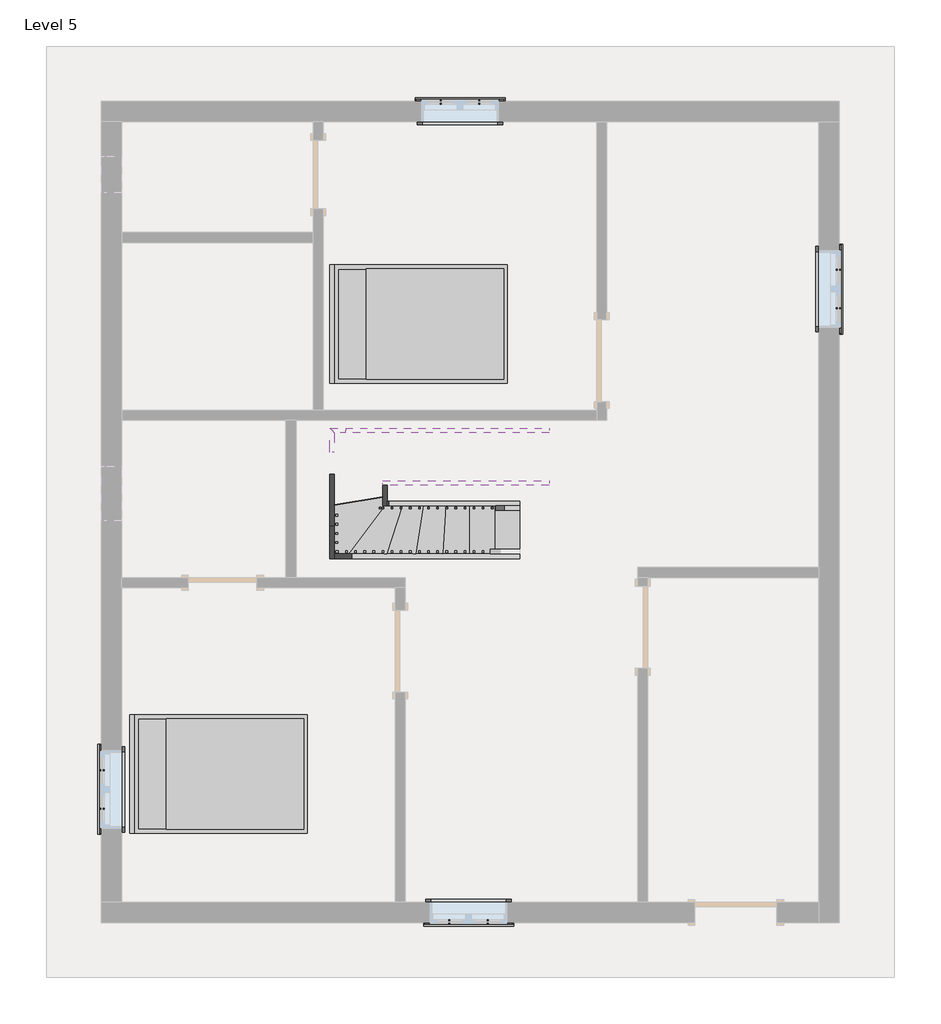
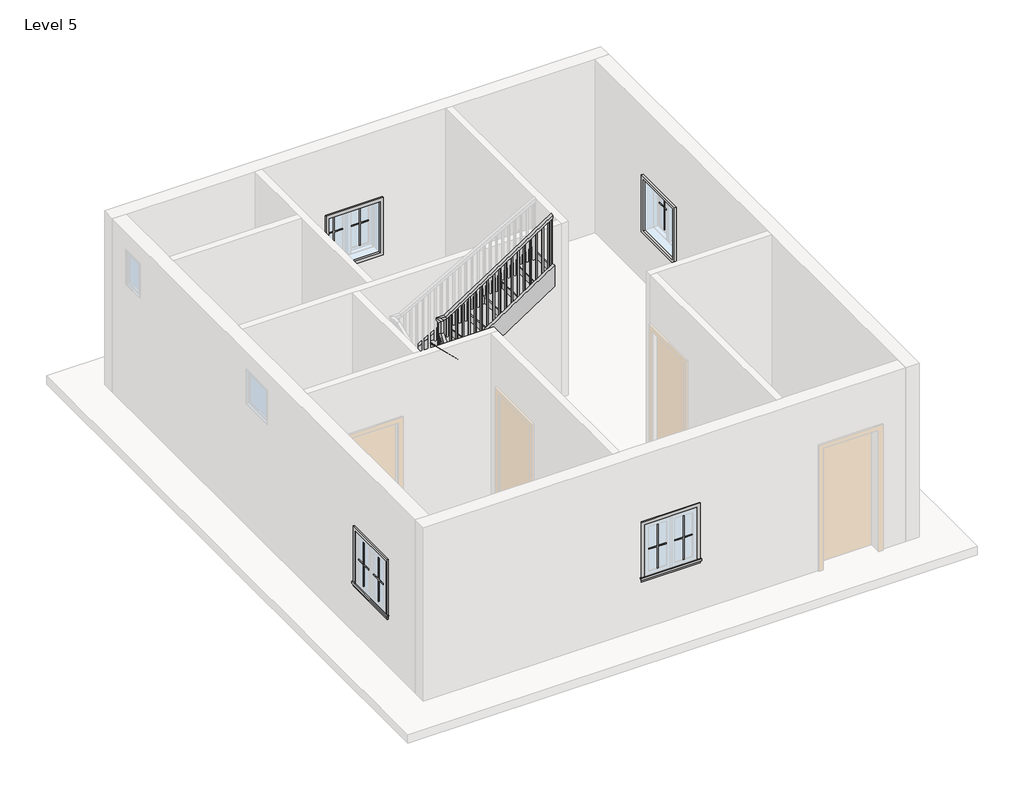
# One storey, part 2 of 2: 16 proxies, 9 members, 2 furniture elements, 1 railing, 1 stair flight.
"""IFC4 building model written with IfcOpenShell, lengths in millimetres."""

from ifc_helpers import new_model, si_unit, frame, origin, place, context, project, spatial, polyline, outline, extrude, faceted_brep, transform, mapped, element, save
from components import muntin_pattern_2x2_muntin_pattern_2x2_b3fe6957, muntin_pattern_2x2_muntin_pattern_2x2_3e0ecaf2, trim_window_exterior_flat_with_sill_41619996, trim_window_interior_flat_picture_frame_51c85655, bed_17739_bed_17739_15c61121, stair_flight_19b8669d

model = new_model("IFC4")

# Units and contexts
model_context = context("Model", 3, world=origin())
ifc_project = project(units=[si_unit("LENGTHUNIT", "METRE", prefix="MILLI")], contexts=[model_context])

# Site, building, storey
site = spatial("IfcSite", under=ifc_project)
building = spatial("IfcBuilding", under=site)
storey = spatial("IfcBuildingStorey", under=building, Name="Level 5", Elevation=9601.2)

# Proxies
placement = place(None, origin())
muntin_pattern_2x2_muntin_pattern_2x2_shape = muntin_pattern_2x2_muntin_pattern_2x2_b3fe6957(model_context)
element("IfcBuildingElementProxy", 1, Name="Muntin Pattern_2x2 : Muntin Pattern_2x2", ObjectType="Muntin Pattern_2x2 : Muntin Pattern_2x2", at=placement, inside=storey, context=model_context, shape_type="MappedRepresentation", body=[
    mapped(muntin_pattern_2x2_muntin_pattern_2x2_shape, transform((-1143.3273498, 4766.5933073, 10585.45), x_axis=(1.0, 0.0, 0.0), y_axis=(0.0, 1.0, 0.0), z_axis=(0.0, 0.0, 1.0))),
])
element("IfcBuildingElementProxy", 2, Name="Muntin Pattern_2x2 : Muntin Pattern_2x2", ObjectType="Muntin Pattern_2x2 : Muntin Pattern_2x2", at=placement, inside=storey, context=model_context, shape_type="MappedRepresentation", body=[
    mapped(muntin_pattern_2x2_muntin_pattern_2x2_shape, transform((3290.5601502, 2894.9308073, 10585.45), x_axis=(0.0, -1.0, 0.0), y_axis=(1.0, 0.0, 0.0), z_axis=(0.0, 0.0, 1.0))),
])
element("IfcBuildingElementProxy", 3, Name="Muntin Pattern_2x2 : Muntin Pattern_2x2", ObjectType="Muntin Pattern_2x2 : Muntin Pattern_2x2", at=placement, inside=storey, context=model_context, shape_type="MappedRepresentation", body=[
    mapped(muntin_pattern_2x2_muntin_pattern_2x2_shape, transform((-619.4523498, -4374.2316927, 10585.45), x_axis=(-1.0, 0.0, 0.0), y_axis=(0.0, -1.0, 0.0), z_axis=(0.0, 0.0, 1.0))),
])
element("IfcBuildingElementProxy", 4, Name="Muntin Pattern_2x2 : Muntin Pattern_2x2", ObjectType="Muntin Pattern_2x2 : Muntin Pattern_2x2", at=placement, inside=storey, context=model_context, shape_type="MappedRepresentation", body=[
    mapped(muntin_pattern_2x2_muntin_pattern_2x2_shape, transform((-4919.9898498, -3112.1691927, 10585.45), x_axis=(0.0, 1.0, 0.0), y_axis=(-1.0, 0.0, 0.0), z_axis=(0.0, 0.0, 1.0))),
])
muntin_pattern_2x2_muntin_pattern_2x2_2_shape = muntin_pattern_2x2_muntin_pattern_2x2_3e0ecaf2(model_context)
element("IfcBuildingElementProxy", 5, Name="Muntin Pattern_2x2 : Muntin Pattern_2x2", ObjectType="Muntin Pattern_2x2 : Muntin Pattern_2x2", at=placement, inside=storey, context=model_context, shape_type="MappedRepresentation", body=[
    mapped(muntin_pattern_2x2_muntin_pattern_2x2_2_shape, transform((-714.7023498, 4766.5933073, 10585.45), x_axis=(-1.0, 0.0, 0.0), y_axis=(0.0, -1.0, 0.0), z_axis=(0.0, 0.0, 1.0))),
])
element("IfcBuildingElementProxy", 6, Name="Muntin Pattern_2x2 : Muntin Pattern_2x2", ObjectType="Muntin Pattern_2x2 : Muntin Pattern_2x2", at=placement, inside=storey, context=model_context, shape_type="MappedRepresentation", body=[
    mapped(muntin_pattern_2x2_muntin_pattern_2x2_2_shape, transform((3290.5601502, 2466.3058073, 10585.45), x_axis=(0.0, 1.0, 0.0), y_axis=(-1.0, 0.0, 0.0), z_axis=(0.0, 0.0, 1.0))),
])
element("IfcBuildingElementProxy", 7, Name="Muntin Pattern_2x2 : Muntin Pattern_2x2", ObjectType="Muntin Pattern_2x2 : Muntin Pattern_2x2", at=placement, inside=storey, context=model_context, shape_type="MappedRepresentation", body=[
    mapped(muntin_pattern_2x2_muntin_pattern_2x2_2_shape, transform((-1048.0773498, -4374.2316927, 10585.45), x_axis=(1.0, 0.0, 0.0), y_axis=(0.0, 1.0, 0.0), z_axis=(0.0, 0.0, 1.0))),
])
element("IfcBuildingElementProxy", 8, Name="Muntin Pattern_2x2 : Muntin Pattern_2x2", ObjectType="Muntin Pattern_2x2 : Muntin Pattern_2x2", at=placement, inside=storey, context=model_context, shape_type="MappedRepresentation", body=[
    mapped(muntin_pattern_2x2_muntin_pattern_2x2_2_shape, transform((-4919.9898498, -2683.5441927, 10585.45), x_axis=(0.0, -1.0, 0.0), y_axis=(1.0, 0.0, 0.0), z_axis=(0.0, 0.0, 1.0))),
])
trim_window_exterior_flat_with_sill_shape = trim_window_exterior_flat_with_sill_41619996(model_context)
element("IfcBuildingElementProxy", 9, Name="Trim-Window-Exterior-Flat : with Sill", ObjectType="Trim-Window-Exterior-Flat : with Sill", at=placement, inside=storey, context=model_context, shape_type="MappedRepresentation", body=[
    mapped(trim_window_exterior_flat_with_sill_shape, transform((-929.0148498, 4776.1183073, 11430.0), x_axis=(-1.0, 0.0, 0.0), y_axis=(0.0, 0.0, 1.0), z_axis=(0.0, 1.0, 0.0))),
])
element("IfcBuildingElementProxy", 10, Name="Trim-Window-Exterior-Flat : with Sill", ObjectType="Trim-Window-Exterior-Flat : with Sill", at=placement, inside=storey, context=model_context, shape_type="MappedRepresentation", body=[
    mapped(trim_window_exterior_flat_with_sill_shape, transform((3300.0851502, 2680.6183073, 11430.0), x_axis=(0.0, 1.0, 0.0), y_axis=(0.0, 0.0, 1.0), z_axis=(1.0, 0.0, 0.0))),
])
element("IfcBuildingElementProxy", 11, Name="Trim-Window-Exterior-Flat : with Sill", ObjectType="Trim-Window-Exterior-Flat : with Sill", at=placement, inside=storey, context=model_context, shape_type="MappedRepresentation", body=[
    mapped(trim_window_exterior_flat_with_sill_shape, transform((-833.7648498, -4383.7566927, 11430.0), x_axis=(1.0, 0.0, 0.0), y_axis=(0.0, 0.0, 1.0), z_axis=(0.0, -1.0, 0.0))),
])
element("IfcBuildingElementProxy", 12, Name="Trim-Window-Exterior-Flat : with Sill", ObjectType="Trim-Window-Exterior-Flat : with Sill", at=placement, inside=storey, context=model_context, shape_type="MappedRepresentation", body=[
    mapped(trim_window_exterior_flat_with_sill_shape, transform((-4929.5148498, -2897.8566927, 11430.0), x_axis=(0.0, -1.0, 0.0), y_axis=(0.0, 0.0, 1.0), z_axis=(-1.0, 0.0, 0.0))),
])
trim_window_interior_flat_picture_frame_shape = trim_window_interior_flat_picture_frame_51c85655(model_context)
element("IfcBuildingElementProxy", 13, Name="Trim-Window-Interior-Flat : Picture Frame", ObjectType="Trim-Window-Interior-Flat : Picture Frame", at=placement, inside=storey, context=model_context, shape_type="MappedRepresentation", body=[
    mapped(trim_window_interior_flat_picture_frame_shape, transform((-929.0148498, 4547.5183073, 11430.0), x_axis=(1.0, 0.0, 0.0), y_axis=(0.0, 0.0, 1.0), z_axis=(0.0, -1.0, 0.0))),
])
element("IfcBuildingElementProxy", 14, Name="Trim-Window-Interior-Flat : Picture Frame", ObjectType="Trim-Window-Interior-Flat : Picture Frame", at=placement, inside=storey, context=model_context, shape_type="MappedRepresentation", body=[
    mapped(trim_window_interior_flat_picture_frame_shape, transform((3071.4851502, 2680.6183073, 11430.0), x_axis=(0.0, -1.0, 0.0), y_axis=(0.0, 0.0, 1.0), z_axis=(-1.0, 0.0, 0.0))),
])
element("IfcBuildingElementProxy", 15, Name="Trim-Window-Interior-Flat : Picture Frame", ObjectType="Trim-Window-Interior-Flat : Picture Frame", at=placement, inside=storey, context=model_context, shape_type="MappedRepresentation", body=[
    mapped(trim_window_interior_flat_picture_frame_shape, transform((-833.7648498, -4155.1566927, 11430.0), x_axis=(-1.0, 0.0, 0.0), y_axis=(0.0, 0.0, 1.0), z_axis=(0.0, 1.0, 0.0))),
])
element("IfcBuildingElementProxy", 16, Name="Trim-Window-Interior-Flat : Picture Frame", ObjectType="Trim-Window-Interior-Flat : Picture Frame", at=placement, inside=storey, context=model_context, shape_type="MappedRepresentation", body=[
    mapped(trim_window_interior_flat_picture_frame_shape, transform((-4700.9148498, -2897.8566927, 11430.0), x_axis=(0.0, 1.0, 0.0), y_axis=(0.0, 0.0, 1.0), z_axis=(1.0, 0.0, 0.0))),
])

# Furniture
bed_17739_bed_17739_shape = bed_17739_bed_17739_15c61121(model_context)
element("IfcFurniture", 17, ObjectType="Bed_17739 : Bed_17739", at=placement, inside=storey, context=model_context, shape_type="MappedRepresentation", body=[
    mapped(bed_17739_bed_17739_shape, transform((-3596.0148498, -2726.4066927, 9601.2), x_axis=(0.0, 1.0, 0.0), y_axis=(-1.0, 0.0, 0.0), z_axis=(0.0, 0.0, 1.0))),
])
element("IfcFurniture", 18, ObjectType="Bed_17739 : Bed_17739", at=placement, inside=storey, context=model_context, shape_type="MappedRepresentation", body=[
    mapped(bed_17739_bed_17739_shape, transform((-1367.1648498, 2290.0933073, 9601.2), x_axis=(0.0, 1.0, 0.0), y_axis=(-1.0, 0.0, 0.0), z_axis=(0.0, 0.0, 1.0))),
])

# Members
element("IfcMember", 19, ObjectType="Stringer - 2\" Width", at=placement, inside=storey, context=model_context, shape_type="SweptSolid", body=[
    extrude(outline(polyline([(9601.2, -264.8831579), (9829.6652135, -264.8831579), (10905.4576628, -2328.8610857), (10561.7393024, -2328.8610857), (9601.2, -486.0038318), (9601.2, -264.8831579)])), frame((0.0, -322.6029286, 0.0), z_axis=(0.0, 1.0, 0.0), x_axis=(0.0, 0.0, 1.0)), (0.0, 0.0, 1.0), 50.8),
])
element("IfcMember", 20, ObjectType="Stringer - 2\" Width", at=placement, inside=storey, context=model_context, shape_type="SweptSolid", body=[
    extrude(outline(polyline([(-2328.8610857, -322.6029286), (-2379.6610857, -322.6029286), (-2379.6610857, 39.7116887), (-2328.8610857, 39.7116887), (-2328.8610857, -322.6029286)])), frame((0.0, 0.0, 10561.7393024), z_axis=(0.0, 0.0, 1.0), x_axis=(1.0, 0.0, 0.0)), (0.0, 0.0, 1.0), 343.7183604),
])
element("IfcMember", 21, ObjectType="Stringer - 2\" Width", at=placement, inside=storey, context=model_context, shape_type="SweptSolid", body=[
    extrude(outline(polyline([(39.7116887, 10561.7393024), (39.7116887, 10905.4576628), (861.172384, 11245.2948766), (861.172384, 10901.5765162), (39.7116887, 10561.7393024)])), frame((-2379.6610857, 0.0, 0.0), z_axis=(1.0, 0.0, 0.0), x_axis=(0.0, 1.0, 0.0)), (0.0, 0.0, 1.0), 50.8),
])
element("IfcMember", 22, ObjectType="Stringer - 2\" Width", at=placement, inside=storey, context=model_context, shape_type="SweptSolid", body=[
    extrude(outline(polyline([(-2328.8610857, 861.172384), (-2379.6610857, 861.172384), (-2379.6610857, 1130.8895433), (-2328.8610857, 1080.0895433), (-2328.8610857, 861.172384)])), frame((0.0, 0.0, 10907.8790002), z_axis=(0.0, 0.0, 1.0), x_axis=(1.0, 0.0, 0.0)), (0.0, 0.0, 1.0), 329.8531189),
])
element("IfcMember", 23, ObjectType="Stringer - 2\" Width", at=placement, inside=storey, context=model_context, shape_type="SweptSolid", body=[
    extrude(outline(polyline([(-2328.8610857, 1080.0895433), (-2379.6610857, 1130.8895433), (-2203.9193363, 1130.8895433), (-2203.9193363, 1080.0895433), (-2328.8610857, 1080.0895433)])), frame((0.0, 0.0, 10907.8790002), z_axis=(0.0, 0.0, 1.0), x_axis=(1.0, 0.0, 0.0)), (0.0, 0.0, 1.0), 329.8531189),
])
element("IfcMember", 24, ObjectType="Stringer - 2\" Width", at=placement, inside=storey, context=model_context, shape_type="SweptSolid", body=[
    extrude(outline(polyline([(9601.2, -264.8831579), (9798.1581828, -264.8831579), (10817.6545254, -1741.8148498), (10447.2897368, -1741.8148498), (9601.2, -516.0951544), (9601.2, -264.8831579)])), frame((0.0, 264.4433073, 0.0), z_axis=(0.0, 1.0, 0.0), x_axis=(0.0, 0.0, 1.0)), (0.0, 0.0, 1.0), 50.8),
])
element("IfcMember", 25, ObjectType="Stringer - 2\" Width", at=placement, inside=storey, context=model_context, shape_type="SweptSolid", body=[
    extrude(outline(polyline([(264.4433073, 10526.9590756), (264.4433073, 10986.158282), (493.0433073, 11243.7490234), (493.0433073, 10784.549817), (264.4433073, 10526.9590756)])), frame((-1792.6148498, 0.0, 0.0), z_axis=(1.0, 0.0, 0.0), x_axis=(0.0, 1.0, 0.0)), (0.0, 0.0, 1.0), 50.8),
])
element("IfcMember", 26, ObjectType="Stringer - 2\" Width", at=placement, inside=storey, context=model_context, shape_type="SweptSolid", body=[
    extrude(outline(polyline([(11316.8438732, -1792.6148498), (10951.5121415, -1792.6148498), (12177.9313098, 63.4034409), (12543.2630415, 63.4034409), (11316.8438732, -1792.6148498)])), frame((0.0, 493.0433073, 0.0), z_axis=(0.0, 1.0, 0.0), x_axis=(0.0, 0.0, 1.0)), (0.0, 0.0, 1.0), 50.8),
])
element("IfcMember", 27, ObjectType="Stringer - 2\" Width", at=placement, inside=storey, context=model_context, shape_type="SweptSolid", body=[
    extrude(outline(polyline([(11237.732119, -2203.9193363), (10907.8790002, -2203.9193363), (12163.242957, 63.4034409), (12493.0960758, 63.4034409), (11237.732119, -2203.9193363)])), frame((0.0, 1080.0895433, 0.0), z_axis=(0.0, 1.0, 0.0), x_axis=(0.0, 0.0, 1.0)), (0.0, 0.0, 1.0), 50.8),
])

# Railing
element("IfcRailing", 28, ObjectType="Handrail - Rectangular", at=placement, inside=storey, context=model_context, shape_type="SolidModel", body=[
    faceted_brep([(-264.8831579, 213.6433073, 10684.9333333), (-264.8831579, 213.6433073, 10623.6533076), (-264.8831579, 264.4433073, 10623.6533076), (-264.8831579, 264.4433073, 10684.9333333), (-1716.4148498, 213.6433073, 11664.2160626), (-1767.2148498, 213.6433073, 11637.2084974), (-1767.2148498, 264.4433073, 11637.2084974), (-1716.4148498, 264.4433073, 11664.2160626), (-1716.4148498, 213.6433073, 11878.7989826), (-1767.2148498, 213.6433073, 11827.9989826), (-1767.2148498, 264.4433073, 11827.9989826), (-1716.4148498, 264.4433073, 11878.7989826), (-1843.4148498, 213.6433073, 11878.7989826), (-1843.4148498, 213.6433073, 11827.9989826), (-1792.6148498, 264.4433073, 11827.9989826), (-1792.6148498, 264.4433073, 11878.7989826), (-1843.4148498, 340.6433073, 11878.7989826), (-1843.4148498, 363.4803462, 11827.9989826), (-1792.6148498, 363.4803462, 11827.9989826), (-1792.6148498, 340.6433073, 11878.7989826), (-1843.4148498, 467.6433073, 12021.90495), (-1843.4148498, 518.4433073, 12002.6141359), (-1792.6148498, 518.4433073, 12002.6141359), (-1792.6148498, 467.6433073, 12021.90495), (-1843.4148498, 467.6433073, 12233.174751), (-1843.4148498, 518.4433073, 12182.374751), (-1792.6148498, 518.4433073, 12182.374751), (-1792.6148498, 467.6433073, 12233.174751), (-1843.4148498, 594.6433073, 12233.174751), (-1843.4148498, 594.6433073, 12182.374751), (-1792.6148498, 543.8433073, 12182.374751), (-1792.6148498, 543.8433073, 12233.174751), (-1716.4148498, 594.6433073, 12233.174751), (-1701.3097842, 594.6433073, 12182.374751), (-1701.3097842, 543.8433073, 12182.374751), (-1716.4148498, 543.8433073, 12233.174751), (63.4034409, 594.6433073, 13394.2666667), (63.4034409, 543.8433073, 13394.2666667), (63.4034409, 543.8433073, 13333.6126442), (63.4034409, 594.6433073, 13333.6126442)], [[[0, 1, 2, 3]], [[1, 0, 4, 5]], [[2, 1, 5, 6]], [[3, 2, 6, 7]], [[0, 3, 7, 4]], [[5, 4, 8, 9]], [[6, 5, 9, 10]], [[7, 6, 10, 11]], [[4, 7, 11, 8]], [[9, 8, 12, 13]], [[10, 9, 13, 14]], [[11, 10, 14, 15]], [[8, 11, 15, 12]], [[13, 12, 16, 17]], [[14, 13, 17, 18]], [[15, 14, 18, 19]], [[12, 15, 19, 16]], [[17, 16, 20, 21]], [[18, 17, 21, 22]], [[19, 18, 22, 23]], [[16, 19, 23, 20]], [[21, 20, 24, 25]], [[22, 21, 25, 26]], [[23, 22, 26, 27]], [[20, 23, 27, 24]], [[25, 24, 28, 29]], [[26, 25, 29, 30]], [[27, 26, 30, 31]], [[24, 27, 31, 28]], [[29, 28, 32, 33]], [[30, 29, 33, 34]], [[31, 30, 34, 35]], [[28, 31, 35, 32]], [[36, 37, 38, 39]], [[33, 32, 36, 39]], [[34, 33, 39, 38]], [[35, 34, 38, 37]], [[32, 35, 37, 36]]]),
    extrude(outline(polyline([(13305.5000713, 20.3101502), (13293.07251, 1.2601502), (12310.5333333, 1.2601502), (12310.5333333, 20.3101502), (13305.5000713, 20.3101502)])), frame((0.0, 559.7183073, 0.0), z_axis=(0.0, 1.0, 0.0), x_axis=(0.0, 0.0, 1.0)), (0.0, 0.0, 1.0), 19.05),
    extrude(outline(polyline([(13239.2197441, -81.2898498), (13226.7921828, -100.3398498), (12310.5333333, -100.3398498), (12310.5333333, -81.2898498), (13239.2197441, -81.2898498)])), frame((0.0, 559.7183073, 0.0), z_axis=(0.0, 1.0, 0.0), x_axis=(0.0, 0.0, 1.0)), (0.0, 0.0, 1.0), 19.05),
    extrude(outline(polyline([(13172.939417, -182.8898498), (13160.5118556, -201.9398498), (12310.5333333, -201.9398498), (12310.5333333, -182.8898498), (13172.939417, -182.8898498)])), frame((0.0, 559.7183073, 0.0), z_axis=(0.0, 1.0, 0.0), x_axis=(0.0, 0.0, 1.0)), (0.0, 0.0, 1.0), 19.05),
    extrude(outline(polyline([(13106.6590898, -284.4898498), (13094.2315284, -303.5398498), (12141.2, -303.5398498), (12141.2, -284.4898498), (13106.6590898, -284.4898498)])), frame((0.0, 559.7183073, 0.0), z_axis=(0.0, 1.0, 0.0), x_axis=(0.0, 0.0, 1.0)), (0.0, 0.0, 1.0), 19.05),
    extrude(outline(polyline([(13040.3787626, -386.0898498), (13027.9512012, -405.1398498), (12141.2, -405.1398498), (12141.2, -386.0898498), (13040.3787626, -386.0898498)])), frame((0.0, 559.7183073, 0.0), z_axis=(0.0, 1.0, 0.0), x_axis=(0.0, 0.0, 1.0)), (0.0, 0.0, 1.0), 19.05),
    extrude(outline(polyline([(12974.0984354, -487.6898498), (12961.6708741, -506.7398498), (11971.8666667, -506.7398498), (11971.8666667, -487.6898498), (12974.0984354, -487.6898498)])), frame((0.0, 559.7183073, 0.0), z_axis=(0.0, 1.0, 0.0), x_axis=(0.0, 0.0, 1.0)), (0.0, 0.0, 1.0), 19.05),
    extrude(outline(polyline([(12907.8181082, -589.2898498), (12895.3905469, -608.3398498), (11971.8666667, -608.3398498), (11971.8666667, -589.2898498), (12907.8181082, -589.2898498)])), frame((0.0, 559.7183073, 0.0), z_axis=(0.0, 1.0, 0.0), x_axis=(0.0, 0.0, 1.0)), (0.0, 0.0, 1.0), 19.05),
    extrude(outline(polyline([(12841.5377811, -690.8898498), (12829.1102197, -709.9398498), (11971.8666667, -709.9398498), (11971.8666667, -690.8898498), (12841.5377811, -690.8898498)])), frame((0.0, 559.7183073, 0.0), z_axis=(0.0, 1.0, 0.0), x_axis=(0.0, 0.0, 1.0)), (0.0, 0.0, 1.0), 19.05),
    extrude(outline(polyline([(12775.2574539, -792.4898498), (12762.8298925, -811.5398498), (11802.5333333, -811.5398498), (11802.5333333, -792.4898498), (12775.2574539, -792.4898498)])), frame((0.0, 559.7183073, 0.0), z_axis=(0.0, 1.0, 0.0), x_axis=(0.0, 0.0, 1.0)), (0.0, 0.0, 1.0), 19.05),
    extrude(outline(polyline([(12708.9771267, -894.0898498), (12696.5495653, -913.1398498), (11802.5333333, -913.1398498), (11802.5333333, -894.0898498), (12708.9771267, -894.0898498)])), frame((0.0, 559.7183073, 0.0), z_axis=(0.0, 1.0, 0.0), x_axis=(0.0, 0.0, 1.0)), (0.0, 0.0, 1.0), 19.05),
    extrude(outline(polyline([(12642.6967995, -995.6898498), (12630.2692382, -1014.7398498), (11802.5333333, -1014.7398498), (11802.5333333, -995.6898498), (12642.6967995, -995.6898498)])), frame((0.0, 559.7183073, 0.0), z_axis=(0.0, 1.0, 0.0), x_axis=(0.0, 0.0, 1.0)), (0.0, 0.0, 1.0), 19.05),
    extrude(outline(polyline([(12576.4164723, -1097.2898498), (12563.988911, -1116.3398498), (11633.2, -1116.3398498), (11633.2, -1097.2898498), (12576.4164723, -1097.2898498)])), frame((0.0, 559.7183073, 0.0), z_axis=(0.0, 1.0, 0.0), x_axis=(0.0, 0.0, 1.0)), (0.0, 0.0, 1.0), 19.05),
    extrude(outline(polyline([(12510.1361451, -1198.8898498), (12497.7085838, -1217.9398498), (11633.2, -1217.9398498), (11633.2, -1198.8898498), (12510.1361451, -1198.8898498)])), frame((0.0, 559.7183073, 0.0), z_axis=(0.0, 1.0, 0.0), x_axis=(0.0, 0.0, 1.0)), (0.0, 0.0, 1.0), 19.05),
    extrude(outline(polyline([(12443.855818, -1300.4898498), (12431.4282566, -1319.5398498), (11463.8666667, -1319.5398498), (11463.8666667, -1300.4898498), (12443.855818, -1300.4898498)])), frame((0.0, 559.7183073, 0.0), z_axis=(0.0, 1.0, 0.0), x_axis=(0.0, 0.0, 1.0)), (0.0, 0.0, 1.0), 19.05),
    extrude(outline(polyline([(12377.5754908, -1402.0898498), (12365.1479294, -1421.1398498), (11463.8666667, -1421.1398498), (11463.8666667, -1402.0898498), (12377.5754908, -1402.0898498)])), frame((0.0, 559.7183073, 0.0), z_axis=(0.0, 1.0, 0.0), x_axis=(0.0, 0.0, 1.0)), (0.0, 0.0, 1.0), 19.05),
    extrude(outline(polyline([(12311.2951636, -1503.6898498), (12298.8676023, -1522.7398498), (11463.8666667, -1522.7398498), (11463.8666667, -1503.6898498), (12311.2951636, -1503.6898498)])), frame((0.0, 559.7183073, 0.0), z_axis=(0.0, 1.0, 0.0), x_axis=(0.0, 0.0, 1.0)), (0.0, 0.0, 1.0), 19.05),
    extrude(outline(polyline([(12245.0148364, -1605.2898498), (12232.5872751, -1624.3398498), (11294.5333333, -1624.3398498), (11294.5333333, -1605.2898498), (12245.0148364, -1605.2898498)])), frame((0.0, 559.7183073, 0.0), z_axis=(0.0, 1.0, 0.0), x_axis=(0.0, 0.0, 1.0)), (0.0, 0.0, 1.0), 19.05),
    extrude(outline(polyline([(12178.7345092, -1706.8898498), (12166.3069479, -1725.9398498), (11294.5333333, -1725.9398498), (11294.5333333, -1706.8898498), (12178.7345092, -1706.8898498)])), frame((0.0, 559.7183073, 0.0), z_axis=(0.0, 1.0, 0.0), x_axis=(0.0, 0.0, 1.0)), (0.0, 0.0, 1.0), 19.05),
    extrude(outline(polyline([(-1808.4898498, 534.3183073), (-1827.5398498, 534.3183073), (-1827.5398498, 553.3683073), (-1808.4898498, 553.3683073), (-1808.4898498, 534.3183073)])), frame((0.0, 0.0, 11125.2), z_axis=(0.0, 0.0, 1.0), x_axis=(1.0, 0.0, 0.0)), (0.0, 0.0, 1.0), 1057.174751),
    extrude(outline(polyline([(432.7183073, 11906.0176079), (451.7683073, 11927.483503), (451.7683073, 10955.8666667), (432.7183073, 10955.8666667), (432.7183073, 11906.0176079)])), frame((-1827.5398498, 0.0, 0.0), z_axis=(1.0, 0.0, 0.0), x_axis=(0.0, 1.0, 0.0)), (0.0, 0.0, 1.0), 19.05),
    extrude(outline(polyline([(331.1183073, 11791.532834), (350.1683073, 11812.9987291), (350.1683073, 10955.8666667), (331.1183073, 10955.8666667), (331.1183073, 11791.532834)])), frame((-1827.5398498, 0.0, 0.0), z_axis=(1.0, 0.0, 0.0), x_axis=(0.0, 1.0, 0.0)), (0.0, 0.0, 1.0), 19.05),
    extrude(outline(polyline([(-1779.3581579, 248.5683073), (-1779.3581579, 229.5183073), (-1798.4081579, 229.5183073), (-1798.4081579, 248.5683073), (-1779.3581579, 248.5683073)])), frame((0.0, 0.0, 10617.2), z_axis=(0.0, 0.0, 1.0), x_axis=(1.0, 0.0, 0.0)), (0.0, 0.0, 1.0), 1210.7989826),
    extrude(outline(polyline([(11576.8561166, -1677.7581579), (11589.7082893, -1696.8081579), (10617.2, -1696.8081579), (10617.2, -1677.7581579), (11576.8561166, -1677.7581579)])), frame((0.0, 229.5183073, 0.0), z_axis=(0.0, 1.0, 0.0), x_axis=(0.0, 0.0, 1.0)), (0.0, 0.0, 1.0), 19.05),
    extrude(outline(polyline([(11508.3111955, -1576.1581579), (11521.1633682, -1595.2081579), (10617.2, -1595.2081579), (10617.2, -1576.1581579), (11508.3111955, -1576.1581579)])), frame((0.0, 229.5183073, 0.0), z_axis=(0.0, 1.0, 0.0), x_axis=(0.0, 0.0, 1.0)), (0.0, 0.0, 1.0), 19.05),
    extrude(outline(polyline([(11439.7662744, -1474.5581579), (11452.6184472, -1493.6081579), (10447.8666667, -1493.6081579), (10447.8666667, -1474.5581579), (11439.7662744, -1474.5581579)])), frame((0.0, 229.5183073, 0.0), z_axis=(0.0, 1.0, 0.0), x_axis=(0.0, 0.0, 1.0)), (0.0, 0.0, 1.0), 19.05),
    extrude(outline(polyline([(11371.2213533, -1372.9581579), (11384.0735261, -1392.0081579), (10447.8666667, -1392.0081579), (10447.8666667, -1372.9581579), (11371.2213533, -1372.9581579)])), frame((0.0, 229.5183073, 0.0), z_axis=(0.0, 1.0, 0.0), x_axis=(0.0, 0.0, 1.0)), (0.0, 0.0, 1.0), 19.05),
    extrude(outline(polyline([(11302.6764322, -1271.3581579), (11315.528605, -1290.4081579), (10278.5333333, -1290.4081579), (10278.5333333, -1271.3581579), (11302.6764322, -1271.3581579)])), frame((0.0, 229.5183073, 0.0), z_axis=(0.0, 1.0, 0.0), x_axis=(0.0, 0.0, 1.0)), (0.0, 0.0, 1.0), 19.05),
    extrude(outline(polyline([(11234.1315111, -1169.7581579), (11246.9836839, -1188.8081579), (10278.5333333, -1188.8081579), (10278.5333333, -1169.7581579), (11234.1315111, -1169.7581579)])), frame((0.0, 229.5183073, 0.0), z_axis=(0.0, 1.0, 0.0), x_axis=(0.0, 0.0, 1.0)), (0.0, 0.0, 1.0), 19.05),
    extrude(outline(polyline([(11165.58659, -1068.1581579), (11178.4387628, -1087.2081579), (10109.2, -1087.2081579), (10109.2, -1068.1581579), (11165.58659, -1068.1581579)])), frame((0.0, 229.5183073, 0.0), z_axis=(0.0, 1.0, 0.0), x_axis=(0.0, 0.0, 1.0)), (0.0, 0.0, 1.0), 19.05),
    extrude(outline(polyline([(11097.041669, -966.5581579), (11109.8938417, -985.6081579), (10109.2, -985.6081579), (10109.2, -966.5581579), (11097.041669, -966.5581579)])), frame((0.0, 229.5183073, 0.0), z_axis=(0.0, 1.0, 0.0), x_axis=(0.0, 0.0, 1.0)), (0.0, 0.0, 1.0), 19.05),
    extrude(outline(polyline([(11028.4967479, -864.9581579), (11041.3489206, -884.0081579), (10109.2, -884.0081579), (10109.2, -864.9581579), (11028.4967479, -864.9581579)])), frame((0.0, 229.5183073, 0.0), z_axis=(0.0, 1.0, 0.0), x_axis=(0.0, 0.0, 1.0)), (0.0, 0.0, 1.0), 19.05),
    extrude(outline(polyline([(10959.9518268, -763.3581579), (10972.8039995, -782.4081579), (9939.8666667, -782.4081579), (9939.8666667, -763.3581579), (10959.9518268, -763.3581579)])), frame((0.0, 229.5183073, 0.0), z_axis=(0.0, 1.0, 0.0), x_axis=(0.0, 0.0, 1.0)), (0.0, 0.0, 1.0), 19.05),
    extrude(outline(polyline([(10891.4069057, -661.7581579), (10904.2590784, -680.8081579), (9939.8666667, -680.8081579), (9939.8666667, -661.7581579), (10891.4069057, -661.7581579)])), frame((0.0, 229.5183073, 0.0), z_axis=(0.0, 1.0, 0.0), x_axis=(0.0, 0.0, 1.0)), (0.0, 0.0, 1.0), 19.05),
    extrude(outline(polyline([(10822.8619846, -560.1581579), (10835.7141573, -579.2081579), (9939.8666667, -579.2081579), (9939.8666667, -560.1581579), (10822.8619846, -560.1581579)])), frame((0.0, 229.5183073, 0.0), z_axis=(0.0, 1.0, 0.0), x_axis=(0.0, 0.0, 1.0)), (0.0, 0.0, 1.0), 19.05),
    extrude(outline(polyline([(10754.3170635, -458.5581579), (10767.1692362, -477.6081579), (9770.5333333, -477.6081579), (9770.5333333, -458.5581579), (10754.3170635, -458.5581579)])), frame((0.0, 229.5183073, 0.0), z_axis=(0.0, 1.0, 0.0), x_axis=(0.0, 0.0, 1.0)), (0.0, 0.0, 1.0), 19.05),
    extrude(outline(polyline([(10685.7721424, -356.9581579), (10698.6243151, -376.0081579), (9770.5333333, -376.0081579), (9770.5333333, -356.9581579), (10685.7721424, -356.9581579)])), frame((0.0, 229.5183073, 0.0), z_axis=(0.0, 1.0, 0.0), x_axis=(0.0, 0.0, 1.0)), (0.0, 0.0, 1.0), 19.05),
    extrude(outline(polyline([(-1808.4898498, 559.7183073), (-1827.5398498, 559.7183073), (-1827.5398498, 578.7683073), (-1808.4898498, 578.7683073), (-1808.4898498, 559.7183073)])), frame((0.0, 0.0, 11125.2), z_axis=(0.0, 0.0, 1.0), x_axis=(1.0, 0.0, 0.0)), (0.0, 0.0, 1.0), 1057.174751),
    extrude(outline(polyline([(-1808.4898498, 248.5683073), (-1808.4898498, 229.5183073), (-1827.5398498, 229.5183073), (-1827.5398498, 248.5683073), (-1808.4898498, 248.5683073)])), frame((0.0, 0.0, 10786.5333333), z_axis=(0.0, 0.0, 1.0), x_axis=(1.0, 0.0, 0.0)), (0.0, 0.0, 1.0), 1041.4656493),
    extrude(outline(polyline([(13333.6126442, 63.4034409), (13321.1850828, 44.3534409), (12310.5333333, 44.3534409), (12310.5333333, 63.4034409), (13333.6126442, 63.4034409)])), frame((0.0, 559.7183073, 0.0), z_axis=(0.0, 1.0, 0.0), x_axis=(0.0, 0.0, 1.0)), (0.0, 0.0, 1.0), 19.05),
    extrude(outline(polyline([(10623.6533076, -264.8831579), (10636.5054803, -283.9331579), (9770.5333333, -283.9331579), (9770.5333333, -264.8831579), (10623.6533076, -264.8831579)])), frame((0.0, 229.5183073, 0.0), z_axis=(0.0, 1.0, 0.0), x_axis=(0.0, 0.0, 1.0)), (0.0, 0.0, 1.0), 19.05),
])

# Stair flight
stair_flight_shape = stair_flight_19b8669d(model_context)
element("IfcStairFlight", 29, ObjectType="2\" Tread 1\" Nosing 1/4\" Riser", at=placement, inside=storey, context=model_context, shape_type="MappedRepresentation", body=[
    mapped(stair_flight_shape, transform((0.0, 0.0, 0.0), x_axis=(1.0, 0.0, 0.0), y_axis=(0.0, 1.0, 0.0), z_axis=(0.0, 0.0, 1.0))),
])

save(model, "model.ifc")

# Revit data of these elements
# Type "Muntin Pattern_2x2 : Muntin Pattern_2x2"
#   Width [instance default] = 4' - 0"
#   Thickness = 0' - 0 1/2"
#   Height [instance default] = 4' - 0"
#   Distance = 0' - 0 3/4"
#   Interior Material [instance default] = none
#   Exterior Material [instance default] = none
#   Default Elevation = 0
# Type "Trim-Window-Exterior-Flat : with Sill"
#   Trim Width = 0' - 2 1/4"
#   Trim Thickness_Picture Frame = 0' - 1 1/4"
#   Trim Thickness_with Sill = 0' - 0 3/4"
#   Sill Thickness = 0' - 1 1/4"
#   Opening Width [instance default] = 2' - 0"
#   Opening Height [instance default] = 3' - 0"
#   Default Elevation = 4' - 0"
#   Sill = yes
#   Picture Frame = no
#   Trim Material [instance default] = none
# Type "Trim-Window-Interior-Flat : Picture Frame"
#   Trim Thickness_Picture Frame = 0' - 1 1/4"
#   Trim Width = 0' - 2 1/4"
#   Trim Thickness_with Sill = 0' - 0 3/4"
#   Sill Thickness = 0' - 1 1/4"
#   Opening Width [instance default] = 2' - 0"
#   Opening Height [instance default] = 3' - 0"
#   Default Elevation = 4' - 0"
#   Sill = no
#   Picture Frame = yes
#   Trim Material [instance default] = none
# Type "Bed_17739 : Bed_17739"
#   Default Elevation = 0
# Type "Handrail - Rectangular"
#   Assembly Code = "C2010400"
#   built-in parameter 1008612 = 0.0416667 (stored number, unit not read)
#   built-in parameter 1008611 = 0.0416667 (stored number, unit not read)
#   built-in parameter 1008609 = 0.333333 (stored number, unit not read)
#   built-in parameter 1008604 = 0.166667 (stored number, unit not read)
#   built-in parameter 1008603 = 0.166667 (stored number, unit not read)
#   Railing Height = 3' - 0"
#   built-in parameter 1008630 = 2
#   built-in parameter 1008610 = 2
#   built-in parameter 1008618 = Baluster - Square : 3/4"
# Elements 1, 2, 3, 4, 5, 6, 7, 8 (IfcBuildingElementProxy, "Muntin Pattern_2x2 : Muntin Pattern_2x2")
#   Width = 0' - 11 5/8"
#   Height = 2' - 6 1/2"
#   Interior Material = Wood - Stained
#   Exterior Material = Clad - White
#   Phase Created = New Construction
#   Materials on its faces: "Clad - White", "Wood - Stained"
# Elements 9, 10, 11, 12 (IfcBuildingElementProxy, "Trim-Window-Exterior-Flat : with Sill")
#   Opening Width = 2' - 10"
#   Opening Height = 3' - 0"
#   Trim Material = Clad - White
#   Phase Created = New Construction
#   Materials on its faces: "Clad - White"
# Elements 13, 14, 15, 16 (IfcBuildingElementProxy, "Trim-Window-Interior-Flat : Picture Frame")
#   Opening Width = 2' - 10"
#   Opening Height = 3' - 0"
#   Trim Material = Wood - Stained
#   Phase Created = New Construction
#   Materials on its faces: "Wood - Stained"
# Elements 17, 18 (IfcFurniture, "Bed_17739 : Bed_17739")
#   Phase Created = New Construction
#   Materials on its faces: "legs", "sheets", "bed frame", "Blanket"
# Elements 19, 20, 21, 22, 23, 24, 25, 26, 27 (IfcMember, "Stringer - 2\" Width")
#   Phase Created = New Construction
# Element 28 (IfcRailing, "Handrail - Rectangular")
#   Phase Created = New Construction
# Element 29 (IfcStairFlight, "2\" Tread 1\" Nosing 1/4\" Riser")
#   Phase Created = New Construction
# Materials
#   "Clad - White": class "Wood", colour RGB 242 242 238, transparency 0, Cost = 0
#   "Wood - Stained": class "Wood", colour RGB 224 178 126, transparency 0, Cost = 0
#   "legs": colour RGB 90 73 37, transparency 0, Cost = 0
#   "sheets": colour RGB 200 195 176, transparency 0, Cost = 0
#   "bed frame": colour RGB 90 73 37, transparency 0, Cost = 0
#   "Blanket": class "System", colour RGB 59 0 1, transparency 0, Cost = 0
